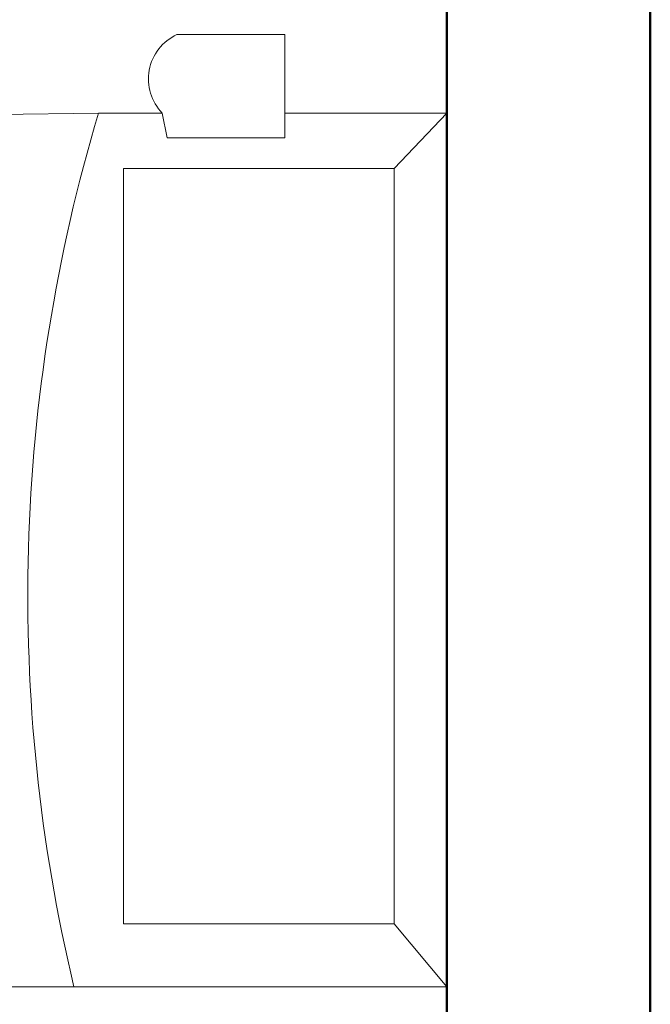
# Model space of a CAD drawing. Units: inches. Extents: x 64 to 1167, y 117 to 939.
# Tile 10 of 56: x 225.92 to 238.33, y 600.21 to 619.57. Entities that reach past the tile are written whole.
import ezdxf

# ---------------------------------------------------------------- set-up
doc = ezdxf.new("R2010")
doc.units = ezdxf.units.IN
doc.header["$MEASUREMENT"] = 0
doc.layers.add('A-FLOR-FIXT', color=8, linetype='Continuous', lineweight=18)
doc.layers.add('A-WALL', color=7, linetype='Continuous', lineweight=50)

# ---------------------------------------------------------------- blocks, each defined once
blk = doc.blocks.new('A$C2B992F40')
for p, q in [((39.23, 615.24), (39.23, 696.15)), ((39.23, 696.15), (475.68, 696.15)), ((66.85, 669.73), (39.23, 696.15)), ((444.23, 669.73), (475.68, 696.15)), ((475.68, 696.15), (475.68, 509.8)), ((66.85, 534.62), (66.85, 669.73)), ((66.85, 669.73), (444.23, 669.73)), ((444.23, 669.73), (444.23, 534.62)), ((0, 561.3), (0, 615.24)), ((0, 615.24), (51.49, 615.24)), ((51.49, 615.24), (51.49, 556.39)), ((51.49, 556.39), (39.23, 553.94)), ((39.23, 522.06), (39.23, 553.94)), ((444.23, 534.62), (66.85, 534.62)), ((40.06, 461.24), (39.23, 522.06)), ((475.68, 509.8), (475.68, 451.92))]:
    blk.add_line(p, q)
for centre, radius, start, end in [((22.2, 571.41), 24.4, 204.4997, 314.261), ((280.26, 1327.83), 841.04, 253.34642, 283.43557)]:
    blk.add_arc(centre, radius, start, end)

msp = doc.modelspace()

# ---------------------------------------------------------------- linework, layer by layer
at = {"layer": 'A-WALL'}
for p, q in [((234.326, 633.2), (234.326, 585.2)), ((238.326, 633.2), (238.326, 585.2))]:
    msp.add_line(p, q, dxfattribs=at)

# ---------------------------------------------------------------- block references
at = {"layer": 'A-FLOR-FIXT', "xscale": 0.0393700787401575, "yscale": 0.0393700787401575, "zscale": 0.0393700787401575, "rotation": 270.0000000000154}
msp.add_blockref('A$C2B992F40', (206.919, 619.278), dxfattribs=at)

doc.saveas('drawing.dxf')
